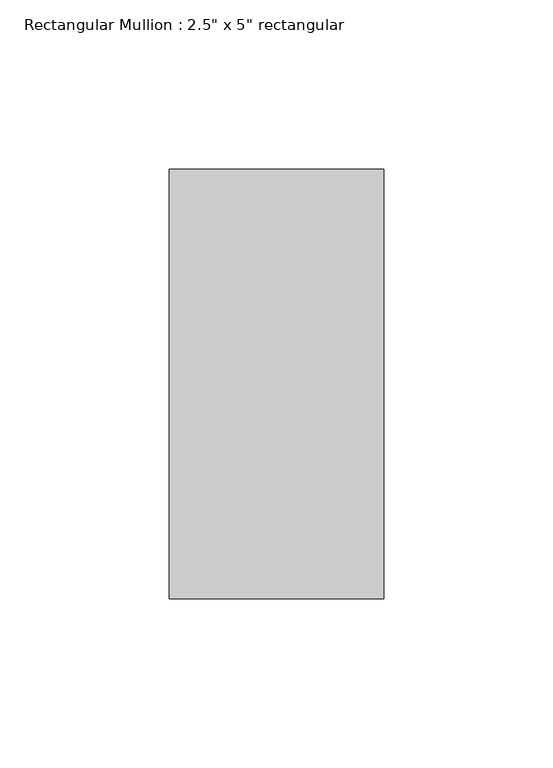
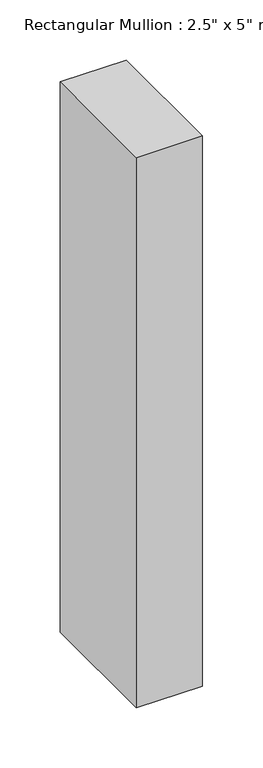
"""IFC4 building model written with IfcOpenShell, lengths in millimetres: member geometry."""

from ifc_helpers import new_model, si_unit, frame, origin, place, context, project, spatial, polyline, outline, extrude, source, transform, mapped, element, save


def member_bc554fa6(model_context):
    return source(origin(), model_context, "Body", "SweptSolid", [
        extrude(outline(polyline([(31.75, 63.5), (31.75, -63.5), (-31.75, -63.5), (-31.75, 63.5), (31.75, 63.5)])), frame((0.0, 0.0, -558.8), z_axis=(0.0, 0.0, 1.0), x_axis=(1.0, 0.0, 0.0)), (0.0, 0.0, 1.0), 558.8),
    ])


if __name__ == "__main__":
    model = new_model("IFC4")
    model_context = context("Model", 3, world=origin())
    ifc_project = project(units=[si_unit("LENGTHUNIT", "METRE", prefix="MILLI")], contexts=[model_context])
    site = spatial("IfcSite", under=ifc_project)
    building = spatial("IfcBuilding", under=site)
    placement = place(None, origin())
    member_shape = member_bc554fa6(model_context)
    element("IfcMember", 1, ObjectType="Rectangular Mullion : 2.5\" x 5\" rectangular", at=placement, inside=building, context=model_context, shape_type="MappedRepresentation", body=[
        mapped(member_shape, transform((0.0, 0.0, 0.0), x_axis=(1.0, 0.0, 0.0), y_axis=(0.0, 1.0, 0.0), z_axis=(0.0, 0.0, 1.0))),
    ])
    save(model, "model.ifc")

# Revit data of these elements
# Type "Rectangular Mullion : 2.5\" x 5\" rectangular"
#   built-in parameter 1007304 = 0.416667 (stored number, unit not read)
#   built-in parameter 1007301 = 0.104167 (stored number, unit not read)
#   built-in parameter 1007300 = 0.104167 (stored number, unit not read)
# Element 1 (IfcMember, "Rectangular Mullion : 2.5\" x 5\" rectangular")
#   Materials on its faces: "Aluminum"
# Materials
#   "Aluminum": class "Metal", colour RGB 247 247 247, transparency 0, Description = "Aluminum 6061", Cost = 0
